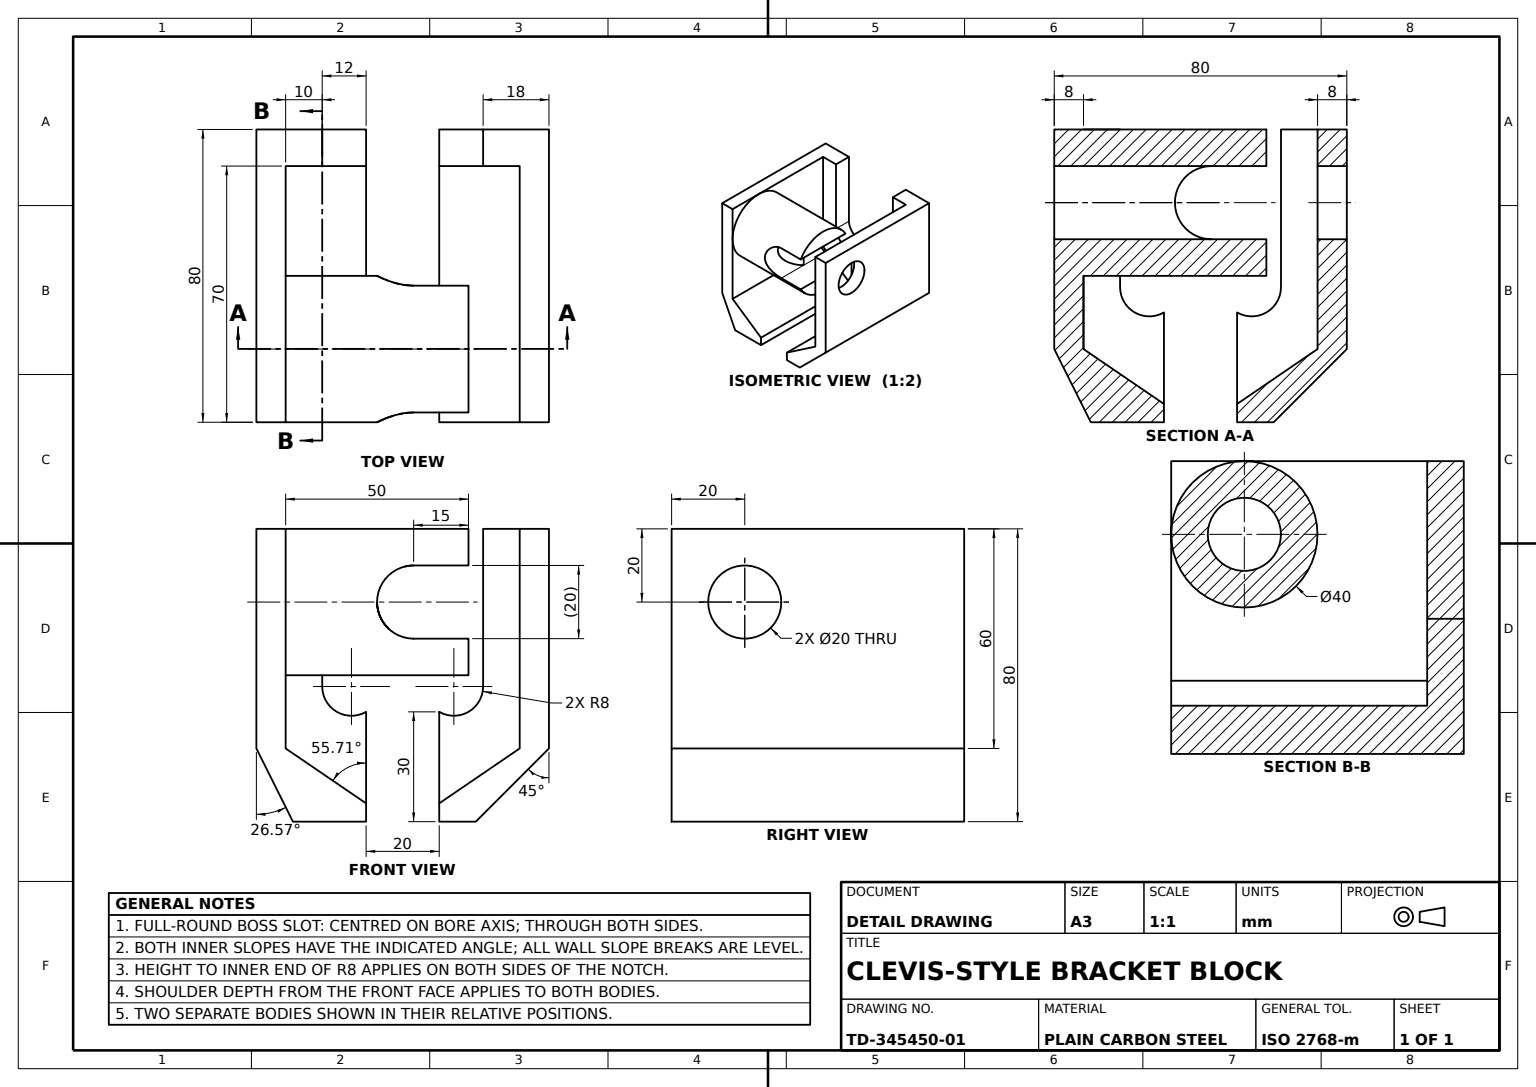
from build123d import *

# Parameters (mm, degrees)
CLEVIS_BODY_DEPTH        = 40
CLEVIS_SLOT_SKETCH_W     = 70
CLEVIS_SLOT_SKETCH_H     = 10
CLEVIS_SLOT_SKETCH_H_2   = 12
CLEVIS_SLOT_CUT_DEPTH    = 60
CLEVIS_RELIEF_CUT_DEPTH  = 70
BRACKET_BODY_DEPTH       = 80
BRACKET_POCKET_CUT_DEPTH = 60
BRACKET_NOTCH_CUT_DEPTH  = 70
PIN_BOSS_SKETCH_R        = 20
PIN_BOSS_DEPTH           = 50
PIN_BOSS_TRIM_CUT_DEPTH  = 50
PIN_HOLE_SKETCH_R        = 10
PIN_HOLE_THROUGH_DEPTH   = 88


with BuildPart() as part:
    # Clevis Body Profile Sketch → Clevis Body (new, symmetric)
    with BuildSketch(Plane(origin=(0, 0, 0), x_dir=(0, 0, -1), z_dir=(1, 0, 0))):
        with BuildLine():
            Line((0, 0), (20, 0))
            Line((20, 0), (30, 20))
            Line((30, 20), (30, 80))
            Line((30, 80), (12, 80))
            Line((12, 80), (12, 36.92820323))
            ThreePointArc((12, 36.92820323), (8, 30), (0, 30))
            Line((0, 30), (0, 0))
        make_face()
    extrude(amount=CLEVIS_BODY_DEPTH, both=True)

    # Clevis Slot Sketch → Clevis Slot Cut (cut)
    with BuildSketch(Plane(origin=(0, 80, 0), x_dir=(1, 0, 0), z_dir=(0, 1, 0))):
        with Locations((-5, 17)):
            Rectangle(CLEVIS_SLOT_SKETCH_W, CLEVIS_SLOT_SKETCH_H)
        with Locations((-5, 6)):
            Rectangle(CLEVIS_SLOT_SKETCH_W, CLEVIS_SLOT_SKETCH_H_2)
    extrude(amount=-CLEVIS_SLOT_CUT_DEPTH, mode=Mode.SUBTRACT)

    # Clevis Relief Sketch → Clevis Relief Cut (cut)
    with BuildSketch(Plane.ZY.offset(40)):
        Polygon((-22, 20), (0, 5), (0, 20), align=None)
    extrude(amount=-CLEVIS_RELIEF_CUT_DEPTH, mode=Mode.SUBTRACT)

    # Pin Boss Sketch → Pin Boss (add)
    with BuildSketch(Plane.XY.offset(-22)):
        with Locations(Location((-20, 60, 0), (0, 0, 180))):
            Circle(PIN_BOSS_SKETCH_R)
    extrude(amount=PIN_BOSS_DEPTH)

    # Pin Boss Trim Sketch → Pin Boss Trim Cut (cut)
    with BuildSketch(Plane(origin=(0, 0, 0), x_dir=(0, 0, -1), z_dir=(1, 0, 0))):
        with BuildLine():
            Line((-13, 70), (-28, 70))
            Line((-28, 70), (-28, 50))
            Line((-28, 50), (-13, 50))
            ThreePointArc((-13, 50), (-3, 60), (-13, 70))
        make_face()
    extrude(amount=-PIN_BOSS_TRIM_CUT_DEPTH, mode=Mode.SUBTRACT)


with BuildPart() as body_2:
    # Bracket Body Profile Sketch → Bracket Body (new body)
    with BuildSketch(Plane(origin=(40, 0, 0), x_dir=(0, 0, -1), z_dir=(1, 0, 0))):
        with BuildLine():
            Line((-30, 0), (-20, 0))
            Line((-20, 0), (-20, 30))
            ThreePointArc((-20, 30), (-28, 30), (-32, 36.92820323))
            Line((-32, 36.92820323), (-32, 80))
            Line((-32, 80), (-50, 80))
            Line((-50, 80), (-50, 20))
            Line((-50, 20), (-30, 0))
        make_face()
    extrude(amount=-BRACKET_BODY_DEPTH)

    # Bracket Pocket Sketch → Bracket Pocket Cut (cut)
    with BuildSketch(Plane(origin=(0, 80, 0), x_dir=(1, 0, 0), z_dir=(0, 1, 0))):
        Polygon((30, -12.853653406), (30, -32), (30, -42), (-40, -42), (-40, -32), (-40, -12.853653406), align=None)
    extrude(amount=-BRACKET_POCKET_CUT_DEPTH, mode=Mode.SUBTRACT)

    # Bracket Notch Sketch → Bracket Notch Cut (cut)
    with BuildSketch(Plane.ZY.offset(40)):
        Polygon((20, 5), (42, 20), (20, 20), align=None)
    extrude(amount=-BRACKET_NOTCH_CUT_DEPTH, mode=Mode.SUBTRACT)


with BuildPart() as pin_hole_through_tool:
    # Pin Hole Sketch → Pin Hole Through (new body)
    with BuildSketch(Plane(origin=(0, 0, -30), x_dir=(-1, 0, 0), z_dir=(0, 0, -1))):
        with Locations((20, 60)):
            Circle(PIN_HOLE_SKETCH_R)
    extrude(amount=-PIN_HOLE_THROUGH_DEPTH)


with BuildPart() as part_1:
    add(part.part)

    # Pin Hole Through: cut by pin_hole_through_tool
    add(pin_hole_through_tool.part, mode=Mode.SUBTRACT)


with BuildPart() as body_2_1:
    add(body_2.part)

    # Pin Hole Through: cut by pin_hole_through_tool
    add(pin_hole_through_tool.part, mode=Mode.SUBTRACT)


solid = Compound([part_1.part, body_2_1.part])
